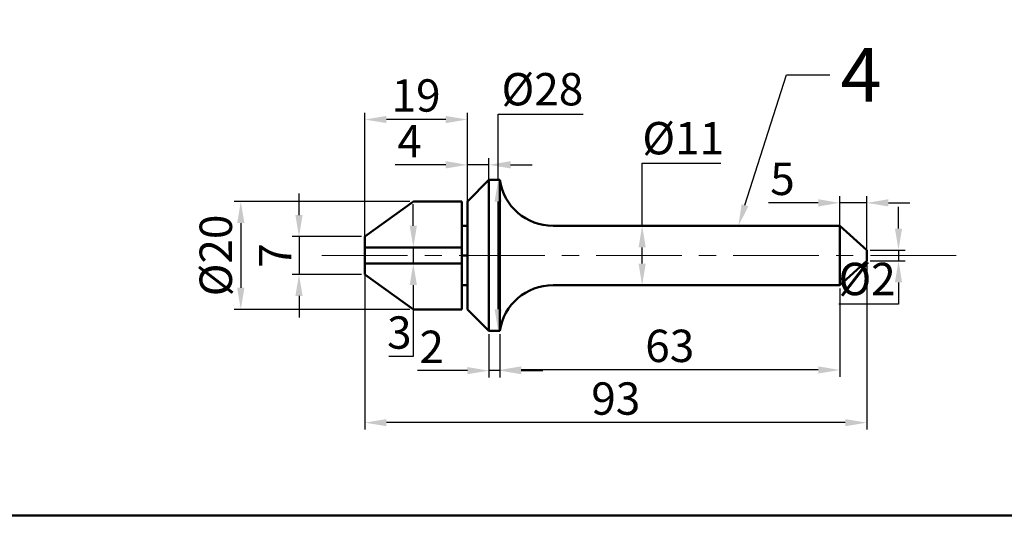
# Model space of a CAD drawing. Units: millimetres. Extents: x -25 to 763, y -62 to 306.
# Tile 2 of 7: x 258 to 440, y -62 to 29. Entities that reach past the tile are written whole.
import ezdxf
from ezdxf import colors
from ezdxf.entities.mleader import LeaderData, LeaderLine
from ezdxf.math import Vec2, Vec3

# ---------------------------------------------------------------- set-up
doc = ezdxf.new("R2010")
doc.units = ezdxf.units.MM
doc.header["$LTSCALE"] = 0.5
doc.linetypes.add('CENTER', pattern=[50.8, 31.75, -6.35, 6.35, -6.35])
for name, color, linetype, lineweight in [('M-CNTR', 1, 'CENTER', 18), ('M-DIMS', 2, 'Continuous', 25), ('M-OUTL', 7, 'Continuous', 50), ('M-TEXT', 3, 'Continuous', 25), ('M-TTLB', 7, 'Continuous', 50)]:
    doc.layers.add(name, color=color, linetype=linetype, lineweight=lineweight)
doc.styles.get("Standard").update_dxf_attribs({"font": 'arial.ttf'})
doc.dimstyles.new('ISO-25', dxfattribs={"dimtxt": 6, "dimasz": 4, "dimexe": 1.25, "dimexo": 0.625, "dimtad": 1, "dimtoh": 1, "dimdec": 1, "dimtxsty": 'Standard', "dimcen": 2.5, "dimadec": 0, "dimazin": 0, "dimtfac": 1, "dimtdec": 1, "dimtmove": 0, "dimatfit": 3, "dimfxl": 1, "dimarcsym": 0})

# ---------------------------------------------------------------- blocks, each defined once
blk = doc.blocks.new('*U42')
at = {"layer": 'M-CNTR', "color": 0, "transparency": 16777216}
blk.add_line((-20.94, 0), (99.67, 0), dxfattribs=at)
blk = doc.blocks.new('*D43')
at = {"layer": 'Defpoints', "color": 0, "ltscale": 0.5, "transparency": 16777216}
for p in [(414.66, -13.26), (414.66, -15.26), (420.54, -15.26)]:
    blk.add_point(p, dxfattribs=at)
at = {"layer": 'M-DIMS', "color": 0, "lineweight": -2, "ltscale": 0.5, "transparency": 16777216}
for p, q in [((420.54, -9.26), (420.54, -5.26)), ((415.28, -13.26), (421.79, -13.26)), ((420.54, -13.26), (420.54, -15.26)), ((415.28, -15.26), (421.79, -15.26)), ((420.54, -19.26), (420.54, -23.26)), ((420.54, -23.26), (409.51, -23.26))]:
    blk.add_line(p, q, dxfattribs=at)
at = {"layer": 'M-DIMS', "color": 0, "ltscale": 0.5, "transparency": 16777216}
for points in [[(419.87, -9.26), (421.2, -9.26), (420.54, -13.26)], [(419.87, -19.26), (421.2, -19.26), (420.54, -15.26)]]:
    blk.add_solid(points, dxfattribs=at)
at = {"layer": 'M-DIMS', "color": 0, "ltscale": 0.5, "transparency": 16777216, "insert": (414.71, -19.4), "char_height": 6, "attachment_point": 5}
blk.add_mtext('%%C2', dxfattribs=at)
blk = doc.blocks.new('*D44')
at = {"layer": 'Defpoints', "color": 0, "ltscale": 0.5, "transparency": 16777216}
for p in [(409.66, -4.5), (409.66, -14.26), (414.66, -14.26)]:
    blk.add_point(p, dxfattribs=at)
at = {"layer": 'M-DIMS', "color": 0, "lineweight": -2, "ltscale": 0.5, "transparency": 16777216}
for p, q in [((409.66, -13.63), (409.66, -3.25)), ((414.66, -13.63), (414.66, -3.25)), ((405.66, -4.5), (396.43, -4.5)), ((414.66, -4.5), (409.66, -4.5)), ((418.66, -4.5), (422.66, -4.5))]:
    blk.add_line(p, q, dxfattribs=at)
at = {"layer": 'M-DIMS', "color": 0, "ltscale": 0.5, "transparency": 16777216}
for points in [[(405.66, -3.84), (405.66, -5.17), (409.66, -4.5)], [(418.66, -3.84), (418.66, -5.17), (414.66, -4.5)]]:
    blk.add_solid(points, dxfattribs=at)
at = {"layer": 'M-DIMS', "color": 0, "ltscale": 0.5, "transparency": 16777216, "insert": (399.04, -0.83), "char_height": 6, "attachment_point": 5}
blk.add_mtext('5', dxfattribs=at)
blk = doc.blocks.new('*D45')
at = {"layer": 'Defpoints', "color": 0, "ltscale": 0.5, "transparency": 16777216}
for p in [(409.66, -19.76), (346.66, -28.26), (346.66, -35.49)]:
    blk.add_point(p, dxfattribs=at)
at = {"layer": 'M-DIMS', "color": 0, "lineweight": -2, "ltscale": 0.5, "transparency": 16777216}
for p, q in [((409.66, -20.38), (409.66, -36.74)), ((346.66, -28.88), (346.66, -36.74)), ((405.66, -35.49), (350.66, -35.49))]:
    blk.add_line(p, q, dxfattribs=at)
at = {"layer": 'M-DIMS', "color": 0, "ltscale": 0.5, "transparency": 16777216}
for points in [[(350.66, -34.82), (350.66, -36.16), (346.66, -35.49)], [(405.66, -34.82), (405.66, -36.16), (409.66, -35.49)]]:
    blk.add_solid(points, dxfattribs=at)
at = {"layer": 'M-DIMS', "color": 0, "ltscale": 0.5, "transparency": 16777216, "insert": (378.16, -31.8), "char_height": 6, "attachment_point": 5}
blk.add_mtext('63', dxfattribs=at)
blk = doc.blocks.new('*D46')
at = {"layer": 'Defpoints', "color": 0, "ltscale": 0.5, "transparency": 16777216}
for p in [(344.66, -28.26), (346.66, -28.26), (344.66, -35.62)]:
    blk.add_point(p, dxfattribs=at)
at = {"layer": 'M-DIMS', "color": 0, "lineweight": -2, "ltscale": 0.5, "transparency": 16777216}
for p, q in [((344.66, -28.88), (344.66, -36.87)), ((346.66, -28.88), (346.66, -36.87)), ((340.66, -35.62), (331.43, -35.62)), ((346.66, -35.62), (344.66, -35.62)), ((350.66, -35.62), (354.66, -35.62))]:
    blk.add_line(p, q, dxfattribs=at)
at = {"layer": 'M-DIMS', "color": 0, "ltscale": 0.5, "transparency": 16777216}
for points in [[(340.66, -34.95), (340.66, -36.28), (344.66, -35.62)], [(350.66, -34.95), (350.66, -36.28), (346.66, -35.62)]]:
    blk.add_solid(points, dxfattribs=at)
at = {"layer": 'M-DIMS', "color": 0, "ltscale": 0.5, "transparency": 16777216, "insert": (334.05, -31.98), "char_height": 6, "attachment_point": 5}
blk.add_mtext('2', dxfattribs=at)
blk = doc.blocks.new('*D47')
at = {"layer": 'Defpoints', "color": 0, "ltscale": 0.5, "transparency": 16777216}
for p in [(340.66, 2.55), (340.66, -8.98), (344.66, -8.98)]:
    blk.add_point(p, dxfattribs=at)
at = {"layer": 'M-DIMS', "color": 0, "lineweight": -2, "ltscale": 0.5, "transparency": 16777216}
for p, q in [((340.66, -8.35), (340.66, 3.8)), ((344.66, -8.35), (344.66, 3.8)), ((336.66, 2.55), (327.26, 2.55)), ((344.66, 2.55), (340.66, 2.55)), ((348.66, 2.55), (352.66, 2.55))]:
    blk.add_line(p, q, dxfattribs=at)
at = {"layer": 'M-DIMS', "color": 0, "ltscale": 0.5, "transparency": 16777216}
for points in [[(336.66, 3.22), (336.66, 1.88), (340.66, 2.55)], [(348.66, 3.22), (348.66, 1.88), (344.66, 2.55)]]:
    blk.add_solid(points, dxfattribs=at)
at = {"layer": 'M-DIMS', "color": 0, "ltscale": 0.5, "transparency": 16777216, "insert": (329.96, 6.17), "char_height": 6, "attachment_point": 5}
blk.add_mtext('4', dxfattribs=at)
blk = doc.blocks.new('*D48')
at = {"layer": 'Defpoints', "color": 0, "ltscale": 0.5, "transparency": 16777216}
for p in [(321.66, 10.95), (321.66, -14.26), (340.66, -14.26)]:
    blk.add_point(p, dxfattribs=at)
at = {"layer": 'M-DIMS', "color": 0, "lineweight": -2, "ltscale": 0.5, "transparency": 16777216}
for p, q in [((321.66, -13.63), (321.66, 12.2)), ((336.66, 10.95), (325.66, 10.95)), ((340.66, -13.63), (340.66, 12.2))]:
    blk.add_line(p, q, dxfattribs=at)
at = {"layer": 'M-DIMS', "color": 0, "ltscale": 0.5, "transparency": 16777216}
for points in [[(325.66, 11.61), (325.66, 10.28), (321.66, 10.95)], [(336.66, 11.61), (336.66, 10.28), (340.66, 10.95)]]:
    blk.add_solid(points, dxfattribs=at)
at = {"layer": 'M-DIMS', "color": 0, "ltscale": 0.5, "transparency": 16777216, "insert": (331.16, 14.63), "char_height": 6, "attachment_point": 5}
blk.add_mtext('19', dxfattribs=at)
blk = doc.blocks.new('*D49')
at = {"layer": 'Defpoints', "color": 0, "ltscale": 0.5, "transparency": 16777216}
for p in [(331.16, -12.76), (330.65, -15.76), (331.16, -15.76)]:
    blk.add_point(p, dxfattribs=at)
at = {"layer": 'M-DIMS', "color": 0, "lineweight": -2, "ltscale": 0.5, "transparency": 16777216}
for p, q in [((330.65, -8.76), (330.65, -4.76)), ((330.53, -12.76), (329.4, -12.76)), ((330.65, -12.76), (330.65, -15.76)), ((330.53, -15.76), (329.4, -15.76)), ((330.65, -19.76), (330.65, -33.02)), ((330.65, -33.02), (326.09, -33.02))]:
    blk.add_line(p, q, dxfattribs=at)
at = {"layer": 'M-DIMS', "color": 0, "ltscale": 0.5, "transparency": 16777216}
for points in [[(329.98, -8.76), (331.31, -8.76), (330.65, -12.76)], [(329.98, -19.76), (331.31, -19.76), (330.65, -15.76)]]:
    blk.add_solid(points, dxfattribs=at)
at = {"layer": 'M-DIMS', "color": 0, "ltscale": 0.5, "transparency": 16777216, "insert": (328.06, -29.33), "char_height": 6, "attachment_point": 5}
blk.add_mtext('3', dxfattribs=at)
blk = doc.blocks.new('*D50')
at = {"layer": 'Defpoints', "color": 0, "ltscale": 0.5, "transparency": 16777216}
for p in [(321.66, -10.76), (309.47, -17.76), (321.66, -17.76)]:
    blk.add_point(p, dxfattribs=at)
at = {"layer": 'M-DIMS', "color": 0, "lineweight": -2, "ltscale": 0.5, "transparency": 16777216}
for p, q in [((309.47, -6.76), (309.47, -2.76)), ((321.03, -10.76), (308.22, -10.76)), ((309.47, -10.76), (309.47, -17.76)), ((321.03, -17.76), (308.22, -17.76)), ((309.47, -21.76), (309.47, -25.76))]:
    blk.add_line(p, q, dxfattribs=at)
at = {"layer": 'M-DIMS', "color": 0, "ltscale": 0.5, "transparency": 16777216}
for points in [[(308.8, -6.76), (310.14, -6.76), (309.47, -10.76)], [(308.8, -21.76), (310.14, -21.76), (309.47, -17.76)]]:
    blk.add_solid(points, dxfattribs=at)
at = {"layer": 'M-DIMS', "color": 0, "ltscale": 0.5, "transparency": 16777216, "insert": (305.84, -14.26), "char_height": 6, "attachment_point": 5, "rotation": 90}
blk.add_mtext('7', dxfattribs=at)
blk = doc.blocks.new('*D51')
at = {"layer": 'Defpoints', "color": 0, "ltscale": 0.5, "transparency": 16777216}
for p in [(330.66, -4.26), (298.69, -24.26), (330.66, -24.26)]:
    blk.add_point(p, dxfattribs=at)
at = {"layer": 'M-DIMS', "color": 0, "lineweight": -2, "ltscale": 0.5, "transparency": 16777216}
for p, q in [((330.03, -4.26), (297.44, -4.26)), ((298.69, -8.26), (298.69, -20.26)), ((330.03, -24.26), (297.44, -24.26))]:
    blk.add_line(p, q, dxfattribs=at)
at = {"layer": 'M-DIMS', "color": 0, "ltscale": 0.5, "transparency": 16777216}
for points in [[(298.02, -8.26), (299.36, -8.26), (298.69, -4.26)], [(298.02, -20.26), (299.36, -20.26), (298.69, -24.26)]]:
    blk.add_solid(points, dxfattribs=at)
at = {"layer": 'M-DIMS', "color": 0, "ltscale": 0.5, "transparency": 16777216, "insert": (294.83, -14.26), "char_height": 6, "attachment_point": 5, "rotation": 90}
blk.add_mtext('%%C20', dxfattribs=at)
blk = doc.blocks.new('*D52')
at = {"layer": 'Defpoints', "color": 0, "ltscale": 0.5, "transparency": 16777216}
for p in [(346.66, -0.26), (346.37, -28.22), (346.66, -28.22)]:
    blk.add_point(p, dxfattribs=at)
at = {"layer": 'M-DIMS', "color": 0, "lineweight": -2, "ltscale": 0.5, "transparency": 16777216}
for p, q in [((346.37, -0.26), (346.37, 11.94)), ((346.37, 11.94), (362.13, 11.94)), ((346.03, -0.26), (345.12, -0.26)), ((346.37, -24.22), (346.37, -4.26)), ((346.03, -28.22), (345.12, -28.22))]:
    blk.add_line(p, q, dxfattribs=at)
at = {"layer": 'M-DIMS', "color": 0, "ltscale": 0.5, "transparency": 16777216}
for points in [[(345.7, -4.26), (347.04, -4.26), (346.37, -0.26)], [(345.7, -24.22), (347.04, -24.22), (346.37, -28.22)]]:
    blk.add_solid(points, dxfattribs=at)
at = {"layer": 'M-DIMS', "color": 0, "ltscale": 0.5, "transparency": 16777216, "insert": (354.56, 15.79), "char_height": 6, "attachment_point": 5}
blk.add_mtext('%%C28', dxfattribs=at)
blk = doc.blocks.new('*D53')
at = {"layer": 'Defpoints', "color": 0, "ltscale": 0.5, "transparency": 16777216}
for p in [(373.04, -8.76), (383.1, -8.76), (383.1, -19.76)]:
    blk.add_point(p, dxfattribs=at)
at = {"layer": 'M-DIMS', "color": 0, "lineweight": -2, "ltscale": 0.5, "transparency": 16777216}
for p, q in [((373.04, -8.76), (373.04, 2.85)), ((373.04, 2.85), (387.63, 2.85)), ((382.47, -8.76), (371.79, -8.76)), ((373.04, -15.76), (373.04, -12.76)), ((382.47, -19.76), (371.79, -19.76))]:
    blk.add_line(p, q, dxfattribs=at)
at = {"layer": 'M-DIMS', "color": 0, "ltscale": 0.5, "transparency": 16777216}
for points in [[(372.38, -12.76), (373.71, -12.76), (373.04, -8.76)], [(372.38, -15.76), (373.71, -15.76), (373.04, -19.76)]]:
    blk.add_solid(points, dxfattribs=at)
at = {"layer": 'M-DIMS', "color": 0, "ltscale": 0.5, "transparency": 16777216, "insert": (380.65, 6.71), "char_height": 6, "attachment_point": 5}
blk.add_mtext('%%C11', dxfattribs=at)
blk = doc.blocks.new('*D54')
at = {"layer": 'Defpoints', "color": 0, "ltscale": 0.5, "transparency": 16777216}
for p in [(321.66, -14.26), (414.66, -14.26), (321.66, -45.26)]:
    blk.add_point(p, dxfattribs=at)
at = {"layer": 'M-DIMS', "color": 0, "lineweight": -2, "ltscale": 0.5, "transparency": 16777216}
for p, q in [((321.66, -14.88), (321.66, -46.51)), ((414.66, -14.88), (414.66, -46.51)), ((410.66, -45.26), (325.66, -45.26))]:
    blk.add_line(p, q, dxfattribs=at)
at = {"layer": 'M-DIMS', "color": 0, "ltscale": 0.5, "transparency": 16777216}
for points in [[(325.66, -44.6), (325.66, -45.93), (321.66, -45.26)], [(410.66, -44.6), (410.66, -45.93), (414.66, -45.26)]]:
    blk.add_solid(points, dxfattribs=at)
at = {"layer": 'M-DIMS', "color": 0, "ltscale": 0.5, "transparency": 16777216, "insert": (368.16, -41.57), "char_height": 6, "attachment_point": 5}
blk.add_mtext('93', dxfattribs=at)

msp = doc.modelspace()

# ---------------------------------------------------------------- linework, layer by layer
at = {"layer": 'M-OUTL', "ltscale": 0.5}
for p, q in [((344.66, -0.26), (340.66, -4.26)), ((344.66, -28.26), (344.66, -0.26)), ((346.66, -0.26), (344.66, -0.26)), ((346.66, -28.26), (346.66, -0.26)), ((339.66, -24.26), (339.66, -4.26)), ((340.66, -24.26), (340.66, -4.26)), ((340.66, -24.26), (340.66, -4.26)), ((340.66, -8.76), (339.66, -8.76)), ((409.66, -8.76), (356.54, -8.76)), ((409.66, -19.76), (409.66, -8.76)), ((409.66, -8.76), (414.66, -13.26)), ((321.66, -10.76), (321.66, -17.76)), ((339.66, -12.76), (321.66, -12.76)), ((340.66, -14.26), (339.66, -14.26)), ((414.66, -14.26), (414.66, -13.26)), ((414.66, -14.26), (414.66, -15.26)), ((339.66, -15.76), (321.66, -15.76)), ((409.66, -19.76), (414.66, -15.26)), ((340.66, -19.76), (339.66, -19.76)), ((356.54, -19.76), (409.66, -19.76)), ((344.66, -28.26), (340.66, -24.26)), ((344.66, -28.26), (346.66, -28.26))]:
    msp.add_line(p, q, dxfattribs=at)
for points in [[(339.66, -4.26), (330.66, -4.26), (321.66, -10.76)], [(321.66, -17.76), (330.66, -24.26), (339.66, -24.26)]]:
    msp.add_lwpolyline(points, dxfattribs=at)
for centre, start, end in [((356.54, 1.24), 188.6269, 270), ((356.54, -29.76), 90, 171.3731)]:
    msp.add_arc(centre, 10, start, end, dxfattribs=at)
at = {"layer": 'M-TTLB', "ltscale": 0.5}
msp.add_lwpolyline([(229.22, 305.74), (763.29, 305.74), (763.29, -62.45), (229.22, -62.45)], close=True, dxfattribs=at)

# ---------------------------------------------------------------- block references
at = {"layer": 'M-CNTR'}
msp.add_blockref('*U42', (334.66, -14.26), dxfattribs=at)

# ---------------------------------------------------------------- dimensions: what is measured, and where the dimension line sits
at = {"layer": 'M-DIMS', "ltscale": 0.5}
for base, p1, p2, picture, middle in [((321.66, 10.95), (340.66, -14.26), (321.66, -14.26), '*D48', (331.16, 14.63)), ((340.66, 2.55), (344.66, -8.98), (340.66, -8.98), '*D47', (329.96, 6.17)), ((409.66, -4.5), (414.66, -14.26), (409.66, -14.26), '*D44', (399.04, -0.83)), ((321.66, -45.26), (414.66, -14.26), (321.66, -14.26), '*D54', (368.16, -41.57)), ((346.66, -35.49), (409.66, -19.76), (346.66, -28.26), '*D45', (378.16, -31.8)), ((344.66, -35.62), (346.66, -28.26), (344.66, -28.26), '*D46', (334.05, -31.98))]:
    dim = msp.add_linear_dim(base=base, p1=p1, p2=p2, dimstyle='ISO-25', override={"dimclrd": 0, "dimclre": 0, "dimclrt": 0}, dxfattribs=at)
    dim.commit()
    dim.dimension.update_dxf_attribs({"geometry": picture, "text_midpoint": middle})
for base, p1, p2, picture, middle in [((346.37, -28.22), (346.66, -0.26), (346.66, -28.22), '*D52', (354.56, 11.94)), ((373.04, -8.76), (383.1, -19.76), (383.1, -8.76), '*D53', (380.65, 2.85)), ((298.69, -24.26), (330.66, -4.26), (330.66, -24.26), '*D51', (298.69, -14.26))]:
    dim = msp.add_linear_dim(base=base, p1=p1, p2=p2, angle=270, text='%%C<>', dimstyle='ISO-25', override={"dimclrd": 0, "dimclre": 0, "dimclrt": 0}, dxfattribs=at)
    dim.commit()
    dim.dimension.update_dxf_attribs({"geometry": picture, "text_midpoint": middle, "dimtype": 160})
for base, p1, p2, picture, middle in [((309.47, -17.76), (321.66, -10.76), (321.66, -17.76), '*D50', (309.47, -14.26)), ((330.65, -15.76), (331.16, -12.76), (331.16, -15.76), '*D49', (328.06, -33.02))]:
    dim = msp.add_linear_dim(base=base, p1=p1, p2=p2, angle=270, dimstyle='ISO-25', override={"dimclrd": 0, "dimclre": 0, "dimclrt": 0}, dxfattribs=at)
    dim.commit()
    dim.dimension.update_dxf_attribs({"geometry": picture, "text_midpoint": middle, "dimtype": 160})
dim = msp.add_linear_dim(base=(420.54, -15.26), p1=(414.66, -13.26), p2=(414.66, -15.26), angle=270, text='%%C<>', dimstyle='ISO-25', override={"dimclrd": 0, "dimclre": 0, "dimclrt": 0}, dxfattribs=at)
dim.commit()
dim.dimension.update_dxf_attribs({"geometry": '*D43', "text_midpoint": (414.71, -19.4)})

# ---------------------------------------------------------------- leaders
at = {"layer": 'M-TEXT', "ltscale": 0.5}
ml = msp.add_multileader_mtext('Standard', dxfattribs=at)
ml.set_content('4', color=256)
ml.set_leader_properties()
ml.build(insert=Vec2(0, 0))
ctx = ml.context
ctx.base_point, ctx.char_height, ctx.plane_origin = Vec3(407.81, 19.23), 10, Vec3(390.88, -8.76)
notes = []
notes.append((ctx, [(0, (1, 1, 0), (399.81, 19.23), (1, 0), 8, [(0, [(390.88, -8.76)], 0, [])])]))
ctx.mtext.insert, ctx.mtext.flow_direction = Vec3(409.81, 24.23), 5
for ctx, leaders in notes:
    for number, flags, end, landing, length, lines in leaders:
        leader = LeaderData()
        leader.index, (leader.has_last_leader_line, leader.has_dogleg_vector, leader.attachment_direction) = number, flags
        leader.last_leader_point, leader.dogleg_vector, leader.dogleg_length = Vec3(end), Vec3(landing), length
        for number, points, colour, breaks in lines:
            line = LeaderLine()
            line.index, line.vertices, line.color, line.breaks = number, Vec3.list(points), colors.encode_raw_color(colour), breaks
            leader.lines.append(line)
        ctx.leaders.append(leader)

doc.saveas('drawing.dxf')
